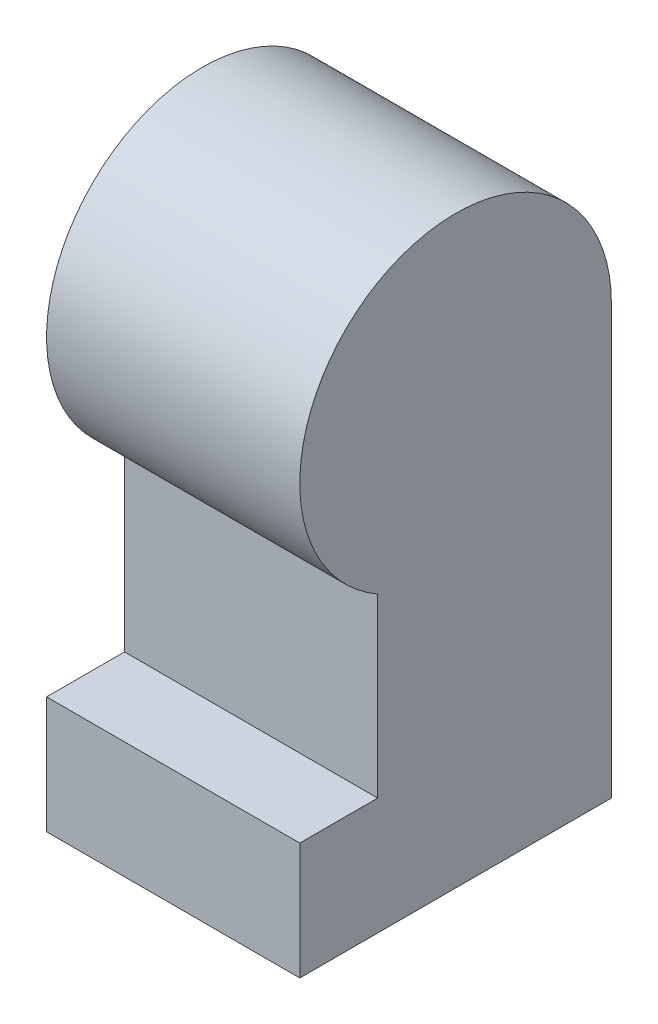
ISO-10303-21;
HEADER;
FILE_DESCRIPTION(('STEP AP214'),'2;1');
FILE_NAME('part.step','',(''),(''),'','','');
FILE_SCHEMA(('AUTOMOTIVE_DESIGN { 1 0 10303 214 1 1 1 1 }'));
ENDSEC;
DATA;
#1=APPLICATION_CONTEXT('core data for automotive mechanical design processes');
#2=APPLICATION_PROTOCOL_DEFINITION('international standard','automotive_design',2000,#1);
#3=PRODUCT_CONTEXT('',#1,'mechanical');
#4=PRODUCT('Part','Part','',(#3));
#5=PRODUCT_RELATED_PRODUCT_CATEGORY('part','',(#4));
#6=PRODUCT_DEFINITION_FORMATION('','',#4);
#7=PRODUCT_DEFINITION_CONTEXT('part definition',#1,'design');
#8=PRODUCT_DEFINITION('design','',#6,#7);
#9=PRODUCT_DEFINITION_SHAPE('','',#8);
#10=(LENGTH_UNIT() NAMED_UNIT(*) SI_UNIT(.MILLI.,.METRE.));
#11=(NAMED_UNIT(*) PLANE_ANGLE_UNIT() SI_UNIT($,.RADIAN.));
#12=(NAMED_UNIT(*) SI_UNIT($,.STERADIAN.) SOLID_ANGLE_UNIT());
#13=UNCERTAINTY_MEASURE_WITH_UNIT(LENGTH_MEASURE(1.E-05),#10,'distance_accuracy_value','');
#14=(GEOMETRIC_REPRESENTATION_CONTEXT(3) GLOBAL_UNCERTAINTY_ASSIGNED_CONTEXT((#13)) GLOBAL_UNIT_ASSIGNED_CONTEXT((#10,
#11,#12)) REPRESENTATION_CONTEXT('',''));
#15=CARTESIAN_POINT('',(0.,0.,0.));
#16=DIRECTION('',(0.,0.,1.));
#17=DIRECTION('',(1.,0.,0.));
#18=AXIS2_PLACEMENT_3D('',#15,#16,#17);
#19=CARTESIAN_POINT('',(3.25,-11.,-4.));
#20=DIRECTION('',(0.,1.,0.));
#21=DIRECTION('',(0.,0.,1.));
#22=AXIS2_PLACEMENT_3D('',#19,#20,#21);
#23=PLANE('',#22);
#24=DIRECTION('',(0.,0.,-1.));
#25=VECTOR('',#24,1.);
#26=CARTESIAN_POINT('',(-3.25,-11.,-4.));
#27=LINE('',#26,#25);
#28=CARTESIAN_POINT('',(-3.25,-11.,4.));
#29=VERTEX_POINT('',#28);
#30=CARTESIAN_POINT('',(-3.25,-11.,-4.));
#31=VERTEX_POINT('',#30);
#32=EDGE_CURVE('E144',#29,#31,#27,.T.);
#33=ORIENTED_EDGE('',*,*,#32,.T.);
#34=DIRECTION('',(-1.,0.,0.));
#35=VECTOR('',#34,1.);
#36=CARTESIAN_POINT('',(3.25,-11.,-4.));
#37=LINE('',#36,#35);
#38=CARTESIAN_POINT('',(3.25,-11.,-4.));
#39=VERTEX_POINT('',#38);
#40=EDGE_CURVE('E126',#39,#31,#37,.T.);
#41=ORIENTED_EDGE('',*,*,#40,.F.);
#42=DIRECTION('',(0.,0.,-1.));
#43=VECTOR('',#42,1.);
#44=CARTESIAN_POINT('',(3.25,-11.,-4.));
#45=LINE('',#44,#43);
#46=CARTESIAN_POINT('',(3.25,-11.,4.));
#47=VERTEX_POINT('',#46);
#48=EDGE_CURVE('E115',#47,#39,#45,.T.);
#49=ORIENTED_EDGE('',*,*,#48,.F.);
#50=DIRECTION('',(-1.,0.,0.));
#51=VECTOR('',#50,1.);
#52=CARTESIAN_POINT('',(3.25,-11.,4.));
#53=LINE('',#52,#51);
#54=EDGE_CURVE('E121',#47,#29,#53,.T.);
#55=ORIENTED_EDGE('',*,*,#54,.T.);
#56=EDGE_LOOP('',(#33,#41,#49,#55));
#57=FACE_BOUND('',#56,.T.);
#58=DIRECTION('',(0.,0.,-1.));
#59=VECTOR('',#58,1.);
#60=CARTESIAN_POINT('',(-2.25,-11.,-4.));
#61=LINE('',#60,#59);
#62=CARTESIAN_POINT('',(-2.25,-11.,3.));
#63=VERTEX_POINT('',#62);
#64=CARTESIAN_POINT('',(-2.25,-11.,-3.));
#65=VERTEX_POINT('',#64);
#66=EDGE_CURVE('E173',#63,#65,#61,.T.);
#67=ORIENTED_EDGE('',*,*,#66,.F.);
#68=DIRECTION('',(-1.,0.,0.));
#69=VECTOR('',#68,1.);
#70=CARTESIAN_POINT('',(3.25,-11.,3.));
#71=LINE('',#70,#69);
#72=CARTESIAN_POINT('',(2.25,-11.,3.));
#73=VERTEX_POINT('',#72);
#74=EDGE_CURVE('E172',#73,#63,#71,.T.);
#75=ORIENTED_EDGE('',*,*,#74,.F.);
#76=DIRECTION('',(0.,0.,-1.));
#77=VECTOR('',#76,1.);
#78=CARTESIAN_POINT('',(2.25,-11.,-4.));
#79=LINE('',#78,#77);
#80=CARTESIAN_POINT('',(2.25,-11.,-3.));
#81=VERTEX_POINT('',#80);
#82=EDGE_CURVE('E53',#73,#81,#79,.T.);
#83=ORIENTED_EDGE('',*,*,#82,.T.);
#84=DIRECTION('',(-1.,0.,0.));
#85=VECTOR('',#84,1.);
#86=CARTESIAN_POINT('',(3.25,-11.,-3.));
#87=LINE('',#86,#85);
#88=EDGE_CURVE('E169',#81,#65,#87,.T.);
#89=ORIENTED_EDGE('',*,*,#88,.T.);
#90=EDGE_LOOP('',(#67,#75,#83,#89));
#91=FACE_BOUND('',#90,.T.);
#92=ADVANCED_FACE('F39',(#57,#91),#23,.F.);
#93=CARTESIAN_POINT('',(3.25,0.,0.));
#94=DIRECTION('',(-1.,0.,0.));
#95=DIRECTION('',(0.,0.,1.));
#96=AXIS2_PLACEMENT_3D('',#93,#94,#95);
#97=CYLINDRICAL_SURFACE('',#96,4.);
#98=CARTESIAN_POINT('',(-3.25,0.,0.));
#99=DIRECTION('',(1.,0.,0.));
#100=DIRECTION('',(0.,0.,-1.));
#101=AXIS2_PLACEMENT_3D('',#98,#99,#100);
#102=CIRCLE('',#101,4.);
#103=CARTESIAN_POINT('',(-3.25,0.,-4.));
#104=VERTEX_POINT('',#103);
#105=CARTESIAN_POINT('',(-3.25,-3.46410161513776,2.));
#106=VERTEX_POINT('',#105);
#107=EDGE_CURVE('E136',#104,#106,#102,.T.);
#108=ORIENTED_EDGE('',*,*,#107,.T.);
#109=DIRECTION('',(-1.,0.,0.));
#110=VECTOR('',#109,1.);
#111=CARTESIAN_POINT('',(3.25,-3.46410161513776,2.));
#112=LINE('',#111,#110);
#113=CARTESIAN_POINT('',(3.25,-3.46410161513776,2.));
#114=VERTEX_POINT('',#113);
#115=EDGE_CURVE('E11',#114,#106,#112,.T.);
#116=ORIENTED_EDGE('',*,*,#115,.F.);
#117=CARTESIAN_POINT('',(3.25,0.,0.));
#118=DIRECTION('',(1.,0.,0.));
#119=DIRECTION('',(0.,0.,-1.));
#120=AXIS2_PLACEMENT_3D('',#117,#118,#119);
#121=CIRCLE('',#120,4.);
#122=CARTESIAN_POINT('',(3.25,0.,-4.));
#123=VERTEX_POINT('',#122);
#124=EDGE_CURVE('E146',#123,#114,#121,.T.);
#125=ORIENTED_EDGE('',*,*,#124,.F.);
#126=DIRECTION('',(-1.,0.,0.));
#127=VECTOR('',#126,1.);
#128=CARTESIAN_POINT('',(3.25,0.,-4.));
#129=LINE('',#128,#127);
#130=EDGE_CURVE('E135',#123,#104,#129,.T.);
#131=ORIENTED_EDGE('',*,*,#130,.T.);
#132=EDGE_LOOP('',(#108,#116,#125,#131));
#133=FACE_BOUND('',#132,.T.);
#134=ADVANCED_FACE('F41',(#133),#97,.T.);
#135=CARTESIAN_POINT('',(3.25,-8.,2.));
#136=DIRECTION('',(0.,0.,-1.));
#137=DIRECTION('',(0.,1.,0.));
#138=AXIS2_PLACEMENT_3D('',#135,#136,#137);
#139=PLANE('',#138);
#140=DIRECTION('',(0.,-1.,0.));
#141=VECTOR('',#140,1.);
#142=CARTESIAN_POINT('',(-3.25,-8.,2.));
#143=LINE('',#142,#141);
#144=CARTESIAN_POINT('',(-3.25,-8.,2.));
#145=VERTEX_POINT('',#144);
#146=EDGE_CURVE('E138',#106,#145,#143,.T.);
#147=ORIENTED_EDGE('',*,*,#146,.T.);
#148=DIRECTION('',(-1.,0.,0.));
#149=VECTOR('',#148,1.);
#150=CARTESIAN_POINT('',(3.25,-8.,2.));
#151=LINE('',#150,#149);
#152=CARTESIAN_POINT('',(3.25,-8.,2.));
#153=VERTEX_POINT('',#152);
#154=EDGE_CURVE('E50',#153,#145,#151,.T.);
#155=ORIENTED_EDGE('',*,*,#154,.F.);
#156=DIRECTION('',(0.,-1.,0.));
#157=VECTOR('',#156,1.);
#158=CARTESIAN_POINT('',(3.25,-8.,2.));
#159=LINE('',#158,#157);
#160=EDGE_CURVE('E98',#114,#153,#159,.T.);
#161=ORIENTED_EDGE('',*,*,#160,.F.);
#162=ORIENTED_EDGE('',*,*,#115,.T.);
#163=EDGE_LOOP('',(#147,#155,#161,#162));
#164=FACE_BOUND('',#163,.T.);
#165=ADVANCED_FACE('F250',(#164),#139,.F.);
#166=CARTESIAN_POINT('',(3.25,-8.,4.));
#167=DIRECTION('',(0.,-1.,0.));
#168=DIRECTION('',(0.,0.,-1.));
#169=AXIS2_PLACEMENT_3D('',#166,#167,#168);
#170=PLANE('',#169);
#171=DIRECTION('',(0.,0.,1.));
#172=VECTOR('',#171,1.);
#173=CARTESIAN_POINT('',(-3.25,-8.,4.));
#174=LINE('',#173,#172);
#175=CARTESIAN_POINT('',(-3.25,-8.,4.));
#176=VERTEX_POINT('',#175);
#177=EDGE_CURVE('E142',#145,#176,#174,.T.);
#178=ORIENTED_EDGE('',*,*,#177,.T.);
#179=DIRECTION('',(-1.,0.,0.));
#180=VECTOR('',#179,1.);
#181=CARTESIAN_POINT('',(3.25,-8.,4.));
#182=LINE('',#181,#180);
#183=CARTESIAN_POINT('',(3.25,-8.,4.));
#184=VERTEX_POINT('',#183);
#185=EDGE_CURVE('E130',#184,#176,#182,.T.);
#186=ORIENTED_EDGE('',*,*,#185,.F.);
#187=DIRECTION('',(0.,0.,1.));
#188=VECTOR('',#187,1.);
#189=CARTESIAN_POINT('',(3.25,-8.,4.));
#190=LINE('',#189,#188);
#191=EDGE_CURVE('E113',#153,#184,#190,.T.);
#192=ORIENTED_EDGE('',*,*,#191,.F.);
#193=ORIENTED_EDGE('',*,*,#154,.T.);
#194=EDGE_LOOP('',(#178,#186,#192,#193));
#195=FACE_BOUND('',#194,.T.);
#196=ADVANCED_FACE('F152',(#195),#170,.F.);
#197=CARTESIAN_POINT('',(3.25,-11.,4.));
#198=DIRECTION('',(0.,0.,-1.));
#199=DIRECTION('',(-1.,0.,0.));
#200=AXIS2_PLACEMENT_3D('',#197,#198,#199);
#201=PLANE('',#200);
#202=DIRECTION('',(0.,-1.,0.));
#203=VECTOR('',#202,1.);
#204=CARTESIAN_POINT('',(-3.25,-11.,4.));
#205=LINE('',#204,#203);
#206=EDGE_CURVE('E123',#176,#29,#205,.T.);
#207=ORIENTED_EDGE('',*,*,#206,.T.);
#208=ORIENTED_EDGE('',*,*,#54,.F.);
#209=DIRECTION('',(0.,-1.,0.));
#210=VECTOR('',#209,1.);
#211=CARTESIAN_POINT('',(3.25,-11.,4.));
#212=LINE('',#211,#210);
#213=EDGE_CURVE('E107',#184,#47,#212,.T.);
#214=ORIENTED_EDGE('',*,*,#213,.F.);
#215=ORIENTED_EDGE('',*,*,#185,.T.);
#216=EDGE_LOOP('',(#207,#208,#214,#215));
#217=FACE_BOUND('',#216,.T.);
#218=ADVANCED_FACE('F122',(#217),#201,.F.);
#219=CARTESIAN_POINT('',(3.25,0.,-4.));
#220=DIRECTION('',(0.,0.,1.));
#221=DIRECTION('',(0.,-1.,0.));
#222=AXIS2_PLACEMENT_3D('',#219,#220,#221);
#223=PLANE('',#222);
#224=DIRECTION('',(0.,1.,0.));
#225=VECTOR('',#224,1.);
#226=CARTESIAN_POINT('',(-3.25,0.,-4.));
#227=LINE('',#226,#225);
#228=EDGE_CURVE('E89',#31,#104,#227,.T.);
#229=ORIENTED_EDGE('',*,*,#228,.T.);
#230=ORIENTED_EDGE('',*,*,#130,.F.);
#231=DIRECTION('',(0.,1.,0.));
#232=VECTOR('',#231,1.);
#233=CARTESIAN_POINT('',(3.25,0.,-4.));
#234=LINE('',#233,#232);
#235=EDGE_CURVE('E63',#39,#123,#234,.T.);
#236=ORIENTED_EDGE('',*,*,#235,.F.);
#237=ORIENTED_EDGE('',*,*,#40,.T.);
#238=EDGE_LOOP('',(#229,#230,#236,#237));
#239=FACE_BOUND('',#238,.T.);
#240=ADVANCED_FACE('F158',(#239),#223,.F.);
#241=CARTESIAN_POINT('',(3.25,0.,0.));
#242=DIRECTION('',(1.,0.,0.));
#243=DIRECTION('',(0.,0.,-1.));
#244=AXIS2_PLACEMENT_3D('',#241,#242,#243);
#245=PLANE('',#244);
#246=ORIENTED_EDGE('',*,*,#124,.T.);
#247=ORIENTED_EDGE('',*,*,#160,.T.);
#248=ORIENTED_EDGE('',*,*,#191,.T.);
#249=ORIENTED_EDGE('',*,*,#213,.T.);
#250=ORIENTED_EDGE('',*,*,#48,.T.);
#251=ORIENTED_EDGE('',*,*,#235,.T.);
#252=EDGE_LOOP('',(#246,#247,#248,#249,#250,#251));
#253=FACE_BOUND('',#252,.T.);
#254=ADVANCED_FACE('F109',(#253),#245,.T.);
#255=CARTESIAN_POINT('',(-3.25,0.,0.));
#256=DIRECTION('',(1.,0.,0.));
#257=DIRECTION('',(0.,0.,-1.));
#258=AXIS2_PLACEMENT_3D('',#255,#256,#257);
#259=PLANE('',#258);
#260=CARTESIAN_POINT('',(-3.25,0.,0.));
#261=DIRECTION('',(-1.,0.,0.));
#262=DIRECTION('',(0.,0.,1.));
#263=AXIS2_PLACEMENT_3D('',#260,#261,#262);
#264=CIRCLE('',#263,1.5);
#265=CARTESIAN_POINT('',(-3.25,0.,1.5));
#266=VERTEX_POINT('',#265);
#267=EDGE_CURVE('E216',#266,#266,#264,.T.);
#268=ORIENTED_EDGE('',*,*,#267,.F.);
#269=EDGE_LOOP('',(#268));
#270=FACE_BOUND('',#269,.T.);
#271=ORIENTED_EDGE('',*,*,#107,.F.);
#272=ORIENTED_EDGE('',*,*,#228,.F.);
#273=ORIENTED_EDGE('',*,*,#32,.F.);
#274=ORIENTED_EDGE('',*,*,#206,.F.);
#275=ORIENTED_EDGE('',*,*,#177,.F.);
#276=ORIENTED_EDGE('',*,*,#146,.F.);
#277=EDGE_LOOP('',(#271,#272,#273,#274,#275,#276));
#278=FACE_BOUND('',#277,.T.);
#279=ADVANCED_FACE('F160',(#270,#278),#259,.F.);
#280=CARTESIAN_POINT('',(3.25,0.,0.));
#281=DIRECTION('',(-1.,0.,0.));
#282=DIRECTION('',(0.,0.,1.));
#283=AXIS2_PLACEMENT_3D('',#280,#281,#282);
#284=CYLINDRICAL_SURFACE('',#283,3.);
#285=CARTESIAN_POINT('',(-2.25,0.,0.));
#286=DIRECTION('',(1.,0.,0.));
#287=DIRECTION('',(0.,0.,-1.));
#288=AXIS2_PLACEMENT_3D('',#285,#286,#287);
#289=CIRCLE('',#288,3.);
#290=CARTESIAN_POINT('',(-2.25,0.,-3.));
#291=VERTEX_POINT('',#290);
#292=CARTESIAN_POINT('',(-2.25,-2.82842712474619,0.999999999999997));
#293=VERTEX_POINT('',#292);
#294=EDGE_CURVE('E206',#291,#293,#289,.T.);
#295=ORIENTED_EDGE('',*,*,#294,.F.);
#296=DIRECTION('',(-1.,0.,0.));
#297=VECTOR('',#296,1.);
#298=CARTESIAN_POINT('',(3.25,0.,-3.));
#299=LINE('',#298,#297);
#300=CARTESIAN_POINT('',(2.25,0.,-3.));
#301=VERTEX_POINT('',#300);
#302=EDGE_CURVE('E175',#301,#291,#299,.T.);
#303=ORIENTED_EDGE('',*,*,#302,.F.);
#304=CARTESIAN_POINT('',(2.25,0.,0.));
#305=DIRECTION('',(1.,0.,0.));
#306=DIRECTION('',(0.,0.,-1.));
#307=AXIS2_PLACEMENT_3D('',#304,#305,#306);
#308=CIRCLE('',#307,3.);
#309=CARTESIAN_POINT('',(2.25,-2.82842712474619,0.999999999999997));
#310=VERTEX_POINT('',#309);
#311=EDGE_CURVE('E181',#301,#310,#308,.T.);
#312=ORIENTED_EDGE('',*,*,#311,.T.);
#313=DIRECTION('',(-1.,0.,0.));
#314=VECTOR('',#313,1.);
#315=CARTESIAN_POINT('',(2.25,-2.82842712474619,0.999999999999997));
#316=LINE('',#315,#314);
#317=EDGE_CURVE('E140',#310,#293,#316,.T.);
#318=ORIENTED_EDGE('',*,*,#317,.T.);
#319=EDGE_LOOP('',(#295,#303,#312,#318));
#320=FACE_BOUND('',#319,.T.);
#321=ADVANCED_FACE('F232',(#320),#284,.F.);
#322=CARTESIAN_POINT('',(3.25,-8.,0.999999999999998));
#323=DIRECTION('',(0.,0.,-1.));
#324=DIRECTION('',(0.,1.,0.));
#325=AXIS2_PLACEMENT_3D('',#322,#323,#324);
#326=PLANE('',#325);
#327=DIRECTION('',(0.,-1.,0.));
#328=VECTOR('',#327,1.);
#329=CARTESIAN_POINT('',(-2.25,-8.,0.999999999999998));
#330=LINE('',#329,#328);
#331=CARTESIAN_POINT('',(-2.25,-9.,0.999999999999998));
#332=VERTEX_POINT('',#331);
#333=EDGE_CURVE('E200',#293,#332,#330,.T.);
#334=ORIENTED_EDGE('',*,*,#333,.F.);
#335=ORIENTED_EDGE('',*,*,#317,.F.);
#336=DIRECTION('',(0.,-1.,0.));
#337=VECTOR('',#336,1.);
#338=CARTESIAN_POINT('',(2.25,-8.,0.999999999999998));
#339=LINE('',#338,#337);
#340=CARTESIAN_POINT('',(2.25,-9.,0.999999999999998));
#341=VERTEX_POINT('',#340);
#342=EDGE_CURVE('E194',#310,#341,#339,.T.);
#343=ORIENTED_EDGE('',*,*,#342,.T.);
#344=DIRECTION('',(-1.,0.,0.));
#345=VECTOR('',#344,1.);
#346=CARTESIAN_POINT('',(3.25,-9.,0.999999999999998));
#347=LINE('',#346,#345);
#348=EDGE_CURVE('E198',#341,#332,#347,.T.);
#349=ORIENTED_EDGE('',*,*,#348,.T.);
#350=EDGE_LOOP('',(#334,#335,#343,#349));
#351=FACE_BOUND('',#350,.T.);
#352=ADVANCED_FACE('F239',(#351),#326,.T.);
#353=CARTESIAN_POINT('',(3.25,-9.,4.));
#354=DIRECTION('',(0.,-1.,0.));
#355=DIRECTION('',(0.,0.,-1.));
#356=AXIS2_PLACEMENT_3D('',#353,#354,#355);
#357=PLANE('',#356);
#358=DIRECTION('',(0.,0.,1.));
#359=VECTOR('',#358,1.);
#360=CARTESIAN_POINT('',(-2.25,-9.,4.));
#361=LINE('',#360,#359);
#362=CARTESIAN_POINT('',(-2.25,-9.,3.));
#363=VERTEX_POINT('',#362);
#364=EDGE_CURVE('E186',#332,#363,#361,.T.);
#365=ORIENTED_EDGE('',*,*,#364,.F.);
#366=ORIENTED_EDGE('',*,*,#348,.F.);
#367=DIRECTION('',(0.,0.,1.));
#368=VECTOR('',#367,1.);
#369=CARTESIAN_POINT('',(2.25,-9.,4.));
#370=LINE('',#369,#368);
#371=CARTESIAN_POINT('',(2.25,-9.,3.));
#372=VERTEX_POINT('',#371);
#373=EDGE_CURVE('E190',#341,#372,#370,.T.);
#374=ORIENTED_EDGE('',*,*,#373,.T.);
#375=DIRECTION('',(-1.,0.,0.));
#376=VECTOR('',#375,1.);
#377=CARTESIAN_POINT('',(3.25,-9.,3.));
#378=LINE('',#377,#376);
#379=EDGE_CURVE('E180',#372,#363,#378,.T.);
#380=ORIENTED_EDGE('',*,*,#379,.T.);
#381=EDGE_LOOP('',(#365,#366,#374,#380));
#382=FACE_BOUND('',#381,.T.);
#383=ADVANCED_FACE('F305',(#382),#357,.T.);
#384=CARTESIAN_POINT('',(3.25,-11.,3.));
#385=DIRECTION('',(0.,0.,-1.));
#386=DIRECTION('',(-1.,0.,0.));
#387=AXIS2_PLACEMENT_3D('',#384,#385,#386);
#388=PLANE('',#387);
#389=DIRECTION('',(0.,-1.,0.));
#390=VECTOR('',#389,1.);
#391=CARTESIAN_POINT('',(-2.25,-11.,3.));
#392=LINE('',#391,#390);
#393=EDGE_CURVE('E177',#363,#63,#392,.T.);
#394=ORIENTED_EDGE('',*,*,#393,.F.);
#395=ORIENTED_EDGE('',*,*,#379,.F.);
#396=DIRECTION('',(0.,-1.,0.));
#397=VECTOR('',#396,1.);
#398=CARTESIAN_POINT('',(2.25,-11.,3.));
#399=LINE('',#398,#397);
#400=EDGE_CURVE('E170',#372,#73,#399,.T.);
#401=ORIENTED_EDGE('',*,*,#400,.T.);
#402=ORIENTED_EDGE('',*,*,#74,.T.);
#403=EDGE_LOOP('',(#394,#395,#401,#402));
#404=FACE_BOUND('',#403,.T.);
#405=ADVANCED_FACE('F312',(#404),#388,.T.);
#406=CARTESIAN_POINT('',(3.25,0.,-3.));
#407=DIRECTION('',(0.,0.,1.));
#408=DIRECTION('',(0.,-1.,0.));
#409=AXIS2_PLACEMENT_3D('',#406,#407,#408);
#410=PLANE('',#409);
#411=DIRECTION('',(0.,1.,0.));
#412=VECTOR('',#411,1.);
#413=CARTESIAN_POINT('',(-2.25,0.,-3.));
#414=LINE('',#413,#412);
#415=EDGE_CURVE('E176',#65,#291,#414,.T.);
#416=ORIENTED_EDGE('',*,*,#415,.F.);
#417=ORIENTED_EDGE('',*,*,#88,.F.);
#418=DIRECTION('',(0.,1.,0.));
#419=VECTOR('',#418,1.);
#420=CARTESIAN_POINT('',(2.25,0.,-3.));
#421=LINE('',#420,#419);
#422=EDGE_CURVE('E167',#81,#301,#421,.T.);
#423=ORIENTED_EDGE('',*,*,#422,.T.);
#424=ORIENTED_EDGE('',*,*,#302,.T.);
#425=EDGE_LOOP('',(#416,#417,#423,#424));
#426=FACE_BOUND('',#425,.T.);
#427=ADVANCED_FACE('F324',(#426),#410,.T.);
#428=CARTESIAN_POINT('',(2.25,0.,0.));
#429=DIRECTION('',(1.,0.,0.));
#430=DIRECTION('',(0.,0.,-1.));
#431=AXIS2_PLACEMENT_3D('',#428,#429,#430);
#432=PLANE('',#431);
#433=ORIENTED_EDGE('',*,*,#311,.F.);
#434=ORIENTED_EDGE('',*,*,#422,.F.);
#435=ORIENTED_EDGE('',*,*,#82,.F.);
#436=ORIENTED_EDGE('',*,*,#400,.F.);
#437=ORIENTED_EDGE('',*,*,#373,.F.);
#438=ORIENTED_EDGE('',*,*,#342,.F.);
#439=EDGE_LOOP('',(#433,#434,#435,#436,#437,#438));
#440=FACE_BOUND('',#439,.T.);
#441=ADVANCED_FACE('F333',(#440),#432,.F.);
#442=CARTESIAN_POINT('',(-2.25,0.,0.));
#443=DIRECTION('',(1.,0.,0.));
#444=DIRECTION('',(0.,0.,-1.));
#445=AXIS2_PLACEMENT_3D('',#442,#443,#444);
#446=PLANE('',#445);
#447=CARTESIAN_POINT('',(-2.25,0.,0.));
#448=DIRECTION('',(1.,0.,0.));
#449=DIRECTION('',(0.,0.,-1.));
#450=AXIS2_PLACEMENT_3D('',#447,#448,#449);
#451=CIRCLE('',#450,1.5);
#452=CARTESIAN_POINT('',(-2.25,0.,1.5));
#453=VERTEX_POINT('',#452);
#454=EDGE_CURVE('E214',#453,#453,#451,.F.);
#455=ORIENTED_EDGE('',*,*,#454,.T.);
#456=EDGE_LOOP('',(#455));
#457=FACE_BOUND('',#456,.T.);
#458=ORIENTED_EDGE('',*,*,#294,.T.);
#459=ORIENTED_EDGE('',*,*,#333,.T.);
#460=ORIENTED_EDGE('',*,*,#364,.T.);
#461=ORIENTED_EDGE('',*,*,#393,.T.);
#462=ORIENTED_EDGE('',*,*,#66,.T.);
#463=ORIENTED_EDGE('',*,*,#415,.T.);
#464=EDGE_LOOP('',(#458,#459,#460,#461,#462,#463));
#465=FACE_BOUND('',#464,.T.);
#466=ADVANCED_FACE('F225',(#457,#465),#446,.T.);
#467=CARTESIAN_POINT('',(3.251,0.,0.));
#468=DIRECTION('',(-1.,0.,0.));
#469=DIRECTION('',(0.,0.,1.));
#470=AXIS2_PLACEMENT_3D('',#467,#468,#469);
#471=CYLINDRICAL_SURFACE('',#470,1.5);
#472=CARTESIAN_POINT('',(-2.25,0.,1.5));
#473=CARTESIAN_POINT('',(-2.26041666666667,0.,1.5));
#474=CARTESIAN_POINT('',(-2.27083333333333,0.,1.5));
#475=CARTESIAN_POINT('',(-2.29166666666667,0.,1.5));
#476=CARTESIAN_POINT('',(-2.30208333333333,0.,1.5));
#477=CARTESIAN_POINT('',(-2.32291666666667,0.,1.5));
#478=CARTESIAN_POINT('',(-2.33333333333333,0.,1.5));
#479=CARTESIAN_POINT('',(-2.35416666666667,0.,1.5));
#480=CARTESIAN_POINT('',(-2.36458333333333,0.,1.5));
#481=CARTESIAN_POINT('',(-2.38541666666667,0.,1.5));
#482=CARTESIAN_POINT('',(-2.39583333333333,0.,1.5));
#483=CARTESIAN_POINT('',(-2.41666666666667,0.,1.5));
#484=CARTESIAN_POINT('',(-2.42708333333333,0.,1.5));
#485=CARTESIAN_POINT('',(-2.44791666666667,0.,1.5));
#486=CARTESIAN_POINT('',(-2.45833333333333,0.,1.5));
#487=CARTESIAN_POINT('',(-2.47916666666667,0.,1.5));
#488=CARTESIAN_POINT('',(-2.48958333333333,0.,1.5));
#489=CARTESIAN_POINT('',(-2.51041666666667,0.,1.5));
#490=CARTESIAN_POINT('',(-2.52083333333333,0.,1.5));
#491=CARTESIAN_POINT('',(-2.54166666666667,0.,1.5));
#492=CARTESIAN_POINT('',(-2.55208333333333,0.,1.5));
#493=CARTESIAN_POINT('',(-2.57291666666667,0.,1.5));
#494=CARTESIAN_POINT('',(-2.58333333333333,0.,1.5));
#495=CARTESIAN_POINT('',(-2.60416666666667,0.,1.5));
#496=CARTESIAN_POINT('',(-2.61458333333333,0.,1.5));
#497=CARTESIAN_POINT('',(-2.63541666666667,0.,1.5));
#498=CARTESIAN_POINT('',(-2.64583333333333,0.,1.5));
#499=CARTESIAN_POINT('',(-2.66666666666667,0.,1.5));
#500=CARTESIAN_POINT('',(-2.67708333333333,0.,1.5));
#501=CARTESIAN_POINT('',(-2.69791666666667,0.,1.5));
#502=CARTESIAN_POINT('',(-2.70833333333333,0.,1.5));
#503=CARTESIAN_POINT('',(-2.72916666666667,0.,1.5));
#504=CARTESIAN_POINT('',(-2.73958333333333,0.,1.5));
#505=CARTESIAN_POINT('',(-2.76041666666667,0.,1.5));
#506=CARTESIAN_POINT('',(-2.77083333333333,0.,1.5));
#507=CARTESIAN_POINT('',(-2.79166666666667,0.,1.5));
#508=CARTESIAN_POINT('',(-2.80208333333333,0.,1.5));
#509=CARTESIAN_POINT('',(-2.82291666666667,0.,1.5));
#510=CARTESIAN_POINT('',(-2.83333333333333,0.,1.5));
#511=CARTESIAN_POINT('',(-2.85416666666667,0.,1.5));
#512=CARTESIAN_POINT('',(-2.86458333333333,0.,1.5));
#513=CARTESIAN_POINT('',(-2.88541666666667,0.,1.5));
#514=CARTESIAN_POINT('',(-2.89583333333333,0.,1.5));
#515=CARTESIAN_POINT('',(-2.91666666666667,0.,1.5));
#516=CARTESIAN_POINT('',(-2.92708333333333,0.,1.5));
#517=CARTESIAN_POINT('',(-2.94791666666667,0.,1.5));
#518=CARTESIAN_POINT('',(-2.95833333333333,0.,1.5));
#519=CARTESIAN_POINT('',(-2.97916666666667,0.,1.5));
#520=CARTESIAN_POINT('',(-2.98958333333333,0.,1.5));
#521=CARTESIAN_POINT('',(-3.01041666666667,0.,1.5));
#522=CARTESIAN_POINT('',(-3.02083333333333,0.,1.5));
#523=CARTESIAN_POINT('',(-3.04166666666667,0.,1.5));
#524=CARTESIAN_POINT('',(-3.05208333333333,0.,1.5));
#525=CARTESIAN_POINT('',(-3.07291666666667,0.,1.5));
#526=CARTESIAN_POINT('',(-3.08333333333333,0.,1.5));
#527=CARTESIAN_POINT('',(-3.10416666666667,0.,1.5));
#528=CARTESIAN_POINT('',(-3.11458333333333,0.,1.5));
#529=CARTESIAN_POINT('',(-3.13541666666667,0.,1.5));
#530=CARTESIAN_POINT('',(-3.14583333333333,0.,1.5));
#531=CARTESIAN_POINT('',(-3.16666666666667,0.,1.5));
#532=CARTESIAN_POINT('',(-3.17708333333333,0.,1.5));
#533=CARTESIAN_POINT('',(-3.19791666666667,0.,1.5));
#534=CARTESIAN_POINT('',(-3.20833333333333,0.,1.5));
#535=CARTESIAN_POINT('',(-3.22916666666667,0.,1.5));
#536=CARTESIAN_POINT('',(-3.23958333333333,0.,1.5));
#537=CARTESIAN_POINT('',(-3.25,0.,1.5));
#538=B_SPLINE_CURVE_WITH_KNOTS('',3,(#472,#473,#474,#475,#476,#477,#478,#479,#480,#481,#482,
#483,#484,#485,#486,#487,#488,#489,#490,#491,#492,#493,#494,#495,#496,#497,#498,#499,#500,#501,
#502,#503,#504,#505,#506,#507,#508,#509,#510,#511,#512,#513,#514,#515,#516,#517,#518,#519,#520,
#521,#522,#523,#524,#525,#526,#527,#528,#529,#530,#531,#532,#533,#534,#535,#536,#537),
.UNSPECIFIED.,.F.,.F.,(4,2,2,2,2,2,2,2,2,2,2,2,2,2,2,2,2,2,2,2,2,2,2,2,2,2,2,2,2,2,2,2,4),(0.,
0.03125,0.0625000000000001,0.0937500000000001,0.125,0.15625,0.1875,0.21875,0.25,
0.281249999999999,0.312499999999999,0.343749999999999,0.374999999999999,0.40625,0.4375,0.46875,
0.5,0.53125,0.5625,0.59375,0.625,0.65625,0.6875,0.718749999999999,0.749999999999999,
0.781249999999999,0.812499999999999,0.843749999999999,0.874999999999999,0.906249999999999,
0.937499999999999,0.968749999999999,0.999999999999999),.UNSPECIFIED.);
#539=EDGE_CURVE('BSEAM223',#453,#266,#538,.T.);
#540=ORIENTED_EDGE('',*,*,#454,.F.);
#541=ORIENTED_EDGE('',*,*,#267,.T.);
#542=ORIENTED_EDGE('',*,*,#539,.T.);
#543=ORIENTED_EDGE('',*,*,#539,.F.);
#544=EDGE_LOOP('',(#540,#542,#541,#543));
#545=FACE_BOUND('',#544,.T.);
#546=ADVANCED_FACE('F223',(#545),#471,.F.);
#547=CLOSED_SHELL('',(#92,#134,#165,#196,#218,#240,#254,#279,#321,#352,#383,#405,#427,#441,#466,#546));
#548=MANIFOLD_SOLID_BREP('B2',#547);
#549=ADVANCED_BREP_SHAPE_REPRESENTATION('',(#18,#548),#14);
#550=SHAPE_DEFINITION_REPRESENTATION(#9,#549);
ENDSEC;
END-ISO-10303-21;
